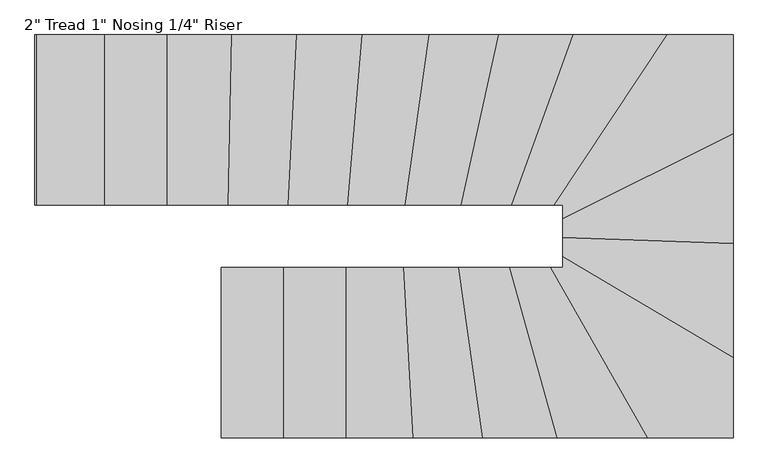
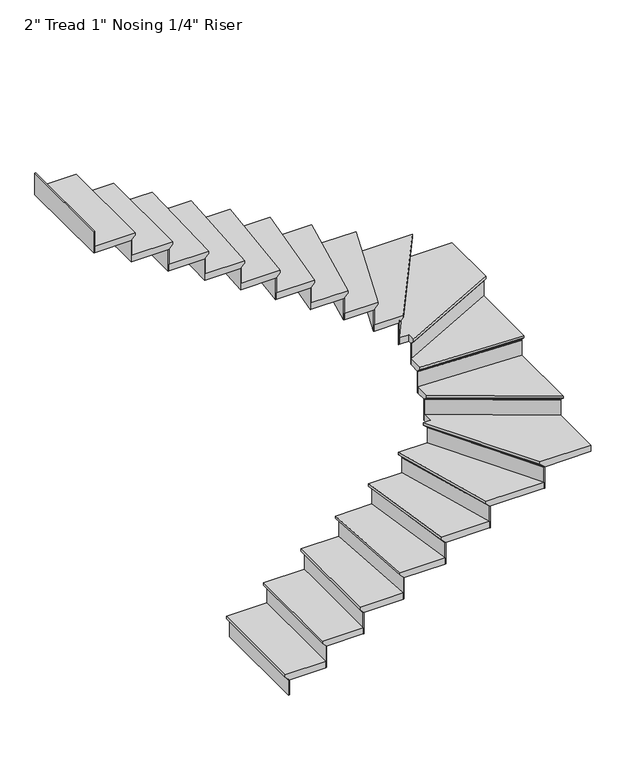
"""IFC4 building model written with IfcOpenShell, lengths in millimetres: stair flight geometry."""

from ifc_helpers import new_model, si_unit, origin, place, context, project, spatial, faceted_brep, source, transform, mapped, element, save


def stair_flight_7608b1ce(model_context):
    return source(origin(), model_context, "Body", "Brep", [
        faceted_brep([(3027.1038904, -664.1159676, 150.2833333), (3027.1038904, -664.1159676, 169.3333333), (3027.1038904, 97.8840324, 169.3333333), (3027.1038904, 97.8840324, 150.2833333), (3052.5038904, -664.1159676, 124.8833333), (3052.5038904, 97.8840324, 124.8833333), (3331.9038904, -664.1159676, 169.3333333), (3331.9038904, 97.8840324, 169.3333333), (3052.5038904, 97.8840324, 118.5333333), (3331.9038904, 97.8840324, 118.5333333), (3331.9038904, -664.1159676, 118.5333333), (3052.5038904, -664.1159676, 118.5333333)], [[[0, 1, 2, 3]], [[4, 0, 3, 5]], [[2, 1, 6, 7]], [[8, 9, 10, 11]], [[2, 7, 9, 8, 5, 3]], [[8, 11, 4, 5]], [[6, 1, 0, 4, 11, 10]], [[7, 6, 10, 9]]]),
        faceted_brep([(3052.5038904, -664.1159676, 118.5333333), (3052.5038904, -664.1159676, 0.0), (3058.8538904, -664.1159676, 0.0), (3058.8538904, -664.1159676, 118.5333333), (3052.5038904, 97.8840324, 118.5333333), (3058.8538904, 97.8840324, 118.5333333), (3058.8538904, 97.8840324, 0.0), (3052.5038904, 97.8840324, 0.0)], [[[0, 1, 2, 3]], [[4, 5, 6, 7]], [[1, 0, 4, 7]], [[2, 1, 7, 6]], [[3, 2, 6, 5]], [[0, 3, 5, 4]]]),
        faceted_brep([(3331.9038904, -664.1159676, 287.8666667), (3331.9038904, -664.1159676, 118.5333333), (3338.2538904, -664.1159676, 118.5333333), (3338.2538904, -664.1159676, 287.8666667), (3331.9038904, 97.8840324, 287.8666667), (3338.2538904, 97.8840324, 287.8666667), (3338.2538904, 97.8840324, 118.5333333), (3331.9038904, 97.8840324, 118.5333333)], [[[0, 1, 2, 3]], [[4, 5, 6, 7]], [[1, 0, 4, 7]], [[2, 1, 7, 6]], [[3, 2, 6, 5]], [[0, 3, 5, 4]]]),
        faceted_brep([(3306.5038904, 97.8840324, 338.6666667), (3306.5038904, -664.1159676, 338.6666667), (3611.3038904, -664.1159676, 338.6666667), (3611.3038904, 97.8840324, 338.6666667), (3331.9038904, 97.8840324, 287.8666667), (3611.3038904, 97.8840324, 287.8666667), (3611.3038904, -664.1159676, 287.8666667), (3331.9038904, -664.1159676, 287.8666667), (3331.9038904, 97.8840324, 294.2166667), (3306.5038904, 97.8840324, 319.6166667), (3331.9038904, -664.1159676, 294.2166667), (3306.5038904, -664.1159676, 319.6166667)], [[[0, 1, 2, 3]], [[4, 5, 6, 7]], [[0, 3, 5, 4, 8, 9]], [[4, 7, 10, 8]], [[2, 1, 11, 10, 7, 6]], [[3, 2, 6, 5]], [[11, 1, 0, 9]], [[10, 11, 9, 8]]]),
        faceted_brep([(3611.3038904, -664.1159676, 457.2), (3611.3038904, -664.1159676, 287.8666667), (3617.6538904, -664.1159676, 287.8666667), (3617.6538904, -664.1159676, 457.2), (3611.3038904, 97.8840324, 457.2), (3617.6538904, 97.8840324, 457.2), (3617.6538904, 97.8840324, 287.8666667), (3611.3038904, 97.8840324, 287.8666667)], [[[0, 1, 2, 3]], [[4, 5, 6, 7]], [[1, 0, 4, 7]], [[2, 1, 7, 6]], [[3, 2, 6, 5]], [[0, 3, 5, 4]]]),
        faceted_brep([(3585.9038904, 97.8840324, 508.0), (3585.9038904, -664.1159676, 508.0), (3912.204517, -664.1159676, 508.0), (3869.2837857, 97.8840324, 508.0), (3611.3038904, 97.8840324, 457.2), (3869.2837857, 97.8840324, 457.2), (3912.204517, -664.1159676, 457.2), (3611.3038904, -664.1159676, 457.2), (3611.3038904, 97.8840324, 463.55), (3585.9038904, 97.8840324, 488.95), (3611.3038904, -664.1159676, 463.55), (3585.9038904, -664.1159676, 488.95)], [[[0, 1, 2, 3]], [[4, 5, 6, 7]], [[0, 3, 5, 4, 8, 9]], [[4, 7, 10, 8]], [[2, 1, 11, 10, 7, 6]], [[3, 2, 6, 5]], [[11, 1, 0, 9]], [[10, 11, 9, 8]]]),
        faceted_brep([(3912.204517, -664.1159676, 626.5333333), (3912.204517, -664.1159676, 457.2), (3918.5645823, -664.1159676, 457.2), (3918.5645823, -664.1159676, 626.5333333), (3869.2837857, 97.8840324, 626.5333333), (3875.6438509, 97.8840324, 626.5333333), (3875.6438509, 97.8840324, 457.2), (3869.2837857, 97.8840324, 457.2)], [[[0, 1, 2, 3]], [[4, 5, 6, 7]], [[1, 0, 4, 7]], [[2, 1, 7, 6]], [[3, 2, 6, 5]], [[0, 3, 5, 4]]]),
        faceted_brep([(3843.8435247, 97.8840324, 677.3333333), (3886.7642561, -664.1159676, 677.3333333), (4223.9651309, -664.1159676, 677.3333333), (4116.7430968, 97.8840324, 677.3333333), (3869.2837857, 97.8840324, 626.5333333), (4116.7430968, 97.8840324, 626.5333333), (4223.9651309, -664.1159676, 626.5333333), (3912.204517, -664.1159676, 626.5333333), (3869.2837857, 97.8840324, 632.8833333), (3843.8435247, 97.8840324, 658.2833333), (3912.204517, -664.1159676, 632.8833333), (3886.7642561, -664.1159676, 658.2833333)], [[[0, 1, 2, 3]], [[4, 5, 6, 7]], [[0, 3, 5, 4, 8, 9]], [[4, 7, 10, 8]], [[2, 1, 11, 10, 7, 6]], [[3, 2, 6, 5]], [[11, 1, 0, 9]], [[10, 11, 9, 8]]]),
        faceted_brep([(4223.9651309, -664.1159676, 795.8666667), (4223.9651309, -664.1159676, 626.5333333), (4230.3776867, -664.1159676, 626.5333333), (4230.3776867, -664.1159676, 795.8666667), (4116.7430968, 97.8840324, 795.8666667), (4123.1556526, 97.8840324, 795.8666667), (4123.1556526, 97.8840324, 626.5333333), (4116.7430968, 97.8840324, 626.5333333)], [[[0, 1, 2, 3]], [[4, 5, 6, 7]], [[1, 0, 4, 7]], [[2, 1, 7, 6]], [[3, 2, 6, 5]], [[0, 3, 5, 4]]]),
        faceted_brep([(4091.0928734, 97.8840324, 846.6666667), (4198.3149075, -664.1159676, 846.6666667), (4557.577462, -664.1159676, 846.6666667), (4343.3988481, 97.8840324, 846.6666667), (4116.7430968, 97.8840324, 795.8666667), (4343.3988481, 97.8840324, 795.8666667), (4557.577462, -664.1159676, 795.8666667), (4223.9651309, -664.1159676, 795.8666667), (4116.7430968, 97.8840324, 802.2166667), (4091.0928734, 97.8840324, 827.6166667), (4223.9651309, -664.1159676, 802.2166667), (4198.3149075, -664.1159676, 827.6166667)], [[[0, 1, 2, 3]], [[4, 5, 6, 7]], [[0, 3, 5, 4, 8, 9]], [[4, 7, 10, 8]], [[2, 1, 11, 10, 7, 6]], [[3, 2, 6, 5]], [[11, 1, 0, 9]], [[10, 11, 9, 8]]]),
        faceted_brep([(4557.577462, -664.1159676, 965.2), (4557.577462, -664.1159676, 795.8666667), (4564.1735282, -664.1159676, 795.8666667), (4564.1735282, -664.1159676, 965.2), (4343.3988481, 97.8840324, 965.2), (4349.9949143, 97.8840324, 965.2), (4349.9949143, 97.8840324, 795.8666667), (4343.3988481, 97.8840324, 795.8666667)], [[[0, 1, 2, 3]], [[4, 5, 6, 7]], [[1, 0, 4, 7]], [[2, 1, 7, 6]], [[3, 2, 6, 5]], [[0, 3, 5, 4]]]),
        faceted_brep([(4317.0145835, 97.8840324, 1016.0), (4531.1931974, -664.1159676, 1016.0), (4964.5066423, -664.1159676, 1016.0), (4531.3858535, 97.8840324, 1016.0), (4343.3988481, 97.8840324, 965.2), (4531.3858535, 97.8840324, 965.2), (4964.5066423, -664.1159676, 965.2), (4557.577462, -664.1159676, 965.2), (4343.3988481, 97.8840324, 971.55), (4317.0145835, 97.8840324, 996.95), (4557.577462, -664.1159676, 971.55), (4531.1931974, -664.1159676, 996.95)], [[[0, 1, 2, 3]], [[4, 5, 6, 7]], [[0, 3, 5, 4, 8, 9]], [[4, 7, 10, 8]], [[2, 1, 11, 10, 7, 6]], [[3, 2, 6, 5]], [[11, 1, 0, 9]], [[10, 11, 9, 8]]]),
        faceted_brep([(4964.5066423, -664.1159676, 1134.5333333), (4964.5066423, -664.1159676, 965.2), (4971.8107395, -664.1159676, 965.2), (4971.8107395, -664.1159676, 1134.5333333), (4531.3858535, 97.8840324, 1134.5333333), (4538.6899506, 97.8840324, 1134.5333333), (4538.6899506, 97.8840324, 965.2), (4531.3858535, 97.8840324, 965.2)], [[[0, 1, 2, 3]], [[4, 5, 6, 7]], [[1, 0, 4, 7]], [[2, 1, 7, 6]], [[3, 2, 6, 5]], [[0, 3, 5, 4]]]),
        faceted_brep([(4554.8355823, 176.4983118, 1185.3333333), (4554.8355823, 97.8840324, 1185.3333333), (4502.1694651, 97.8840324, 1185.3333333), (4935.2902539, -664.1159676, 1185.3333333), (5316.8355823, -664.1159676, 1185.3333333), (5316.8355823, -274.7512133, 1185.3333333), (4554.8355823, 97.8840324, 1134.5333333), (4554.8355823, 176.4983118, 1134.5333333), (5316.8355823, -274.7512133, 1134.5333333), (5316.8355823, -664.1159676, 1134.5333333), (4964.5066423, -664.1159676, 1134.5333333), (4531.3858535, 97.8840324, 1134.5333333), (4531.3858535, 97.8840324, 1140.8833333), (4502.1694651, 97.8840324, 1166.2833333), (4964.5066423, -664.1159676, 1140.8833333), (4935.2902539, -664.1159676, 1166.2833333)], [[[0, 1, 2, 3, 4, 5]], [[6, 7, 8, 9, 10, 11]], [[1, 0, 7, 6]], [[2, 1, 6, 11, 12, 13]], [[11, 10, 14, 12]], [[4, 3, 15, 14, 10, 9]], [[5, 4, 9, 8]], [[0, 5, 8, 7]], [[15, 3, 2, 13]], [[14, 15, 13, 12]]]),
        faceted_brep([(5316.8355823, -274.7512133, 1303.8666667), (5316.8355823, -274.7512133, 1134.5333333), (5316.8355823, -267.3712943, 1134.5333333), (5316.8355823, -267.3712943, 1303.8666667), (4554.8355823, 176.4983118, 1303.8666667), (4554.8355823, 183.8782308, 1303.8666667), (4554.8355823, 183.8782308, 1134.5333333), (4554.8355823, 176.4983118, 1134.5333333)], [[[0, 1, 2, 3]], [[4, 5, 6, 7]], [[1, 0, 4, 7]], [[2, 1, 7, 6]], [[3, 2, 6, 5]], [[0, 3, 5, 4]]]),
        faceted_brep([(4554.8355823, 146.978636, 1354.6666667), (5316.8355823, -304.2708891, 1354.6666667), (5316.8355823, 231.0746698, 1354.6666667), (4554.8355823, 257.0661609, 1354.6666667), (4554.8355823, 176.4983118, 1303.8666667), (4554.8355823, 257.0661609, 1303.8666667), (5316.8355823, 231.0746698, 1303.8666667), (5316.8355823, -274.7512133, 1303.8666667), (4554.8355823, 176.4983118, 1310.2166667), (4554.8355823, 146.978636, 1335.6166667), (5316.8355823, -274.7512133, 1310.2166667), (5316.8355823, -304.2708891, 1335.6166667)], [[[0, 1, 2, 3]], [[4, 5, 6, 7]], [[0, 3, 5, 4, 8, 9]], [[4, 7, 10, 8]], [[3, 2, 6, 5]], [[11, 1, 0, 9]], [[10, 11, 9, 8]], [[2, 1, 11, 10, 7, 6]]]),
        faceted_brep([(5316.8355823, 231.0746698, 1473.2), (5316.8355823, 231.0746698, 1303.8666667), (5316.8355823, 237.4283627, 1303.8666667), (5316.8355823, 237.4283627, 1473.2), (4554.8355823, 257.0661609, 1473.2), (4554.8355823, 263.4198538, 1473.2), (4554.8355823, 263.4198538, 1303.8666667), (4554.8355823, 257.0661609, 1303.8666667)], [[[0, 1, 2, 3]], [[4, 5, 6, 7]], [[1, 0, 4, 7]], [[2, 1, 7, 6]], [[3, 2, 6, 5]], [[0, 3, 5, 4]]]),
        faceted_brep([(4554.8355823, 231.6513892, 1524.0), (5316.8355823, 205.6598981, 1524.0), (5316.8355823, 725.540021, 1524.0), (4554.8355823, 345.3712777, 1524.0), (4554.8355823, 257.0661609, 1473.2), (4554.8355823, 345.3712777, 1473.2), (5316.8355823, 725.540021, 1473.2), (5316.8355823, 231.0746698, 1473.2), (4554.8355823, 257.0661609, 1479.55), (4554.8355823, 231.6513892, 1504.95), (5316.8355823, 231.0746698, 1479.55), (5316.8355823, 205.6598981, 1504.95)], [[[0, 1, 2, 3]], [[4, 5, 6, 7]], [[0, 3, 5, 4, 8, 9]], [[4, 7, 10, 8]], [[2, 1, 11, 10, 7, 6]], [[3, 2, 6, 5]], [[11, 1, 0, 9]], [[10, 11, 9, 8]]]),
        faceted_brep([(5316.8355823, 725.540021, 1642.5333333), (5316.8355823, 725.540021, 1473.2), (5316.8355823, 732.6364416, 1473.2), (5316.8355823, 732.6364416, 1642.5333333), (4554.8355823, 345.3712777, 1642.5333333), (4554.8355823, 352.4676983, 1642.5333333), (4554.8355823, 352.4676983, 1473.2), (4554.8355823, 345.3712777, 1473.2)], [[[0, 1, 2, 3]], [[4, 5, 6, 7]], [[1, 0, 4, 7]], [[2, 1, 7, 6]], [[3, 2, 6, 5]], [[0, 3, 5, 4]]]),
        faceted_brep([(4485.0145037, 377.2840324, 1693.3333333), (4554.8355823, 377.2840324, 1693.3333333), (4554.8355823, 316.9855952, 1693.3333333), (5316.8355823, 697.1543385, 1693.3333333), (5316.8355823, 1139.2840324, 1693.3333333), (4990.2073577, 1139.2840324, 1693.3333333), (4554.8355823, 377.2840324, 1642.5333333), (4485.0145037, 377.2840324, 1642.5333333), (4990.2073577, 1139.2840324, 1642.5333333), (5316.8355823, 1139.2840324, 1642.5333333), (5316.8355823, 725.540021, 1642.5333333), (4554.8355823, 345.3712777, 1642.5333333), (5316.8355823, 725.540021, 1648.8833333), (4554.8355823, 345.3712777, 1648.8833333), (5316.8355823, 697.1543385, 1674.2833333), (4554.8355823, 316.9855952, 1674.2833333)], [[[0, 1, 2, 3, 4, 5]], [[6, 7, 8, 9, 10, 11]], [[1, 0, 7, 6]], [[11, 10, 12, 13]], [[4, 3, 14, 12, 10, 9]], [[5, 4, 9, 8]], [[0, 5, 8, 7]], [[14, 3, 2, 15]], [[12, 14, 15, 13]], [[2, 1, 6, 11, 13, 15]]]),
        faceted_brep([(4990.2073577, 1139.2840324, 1811.8666667), (4990.2073577, 1139.2840324, 1642.5333333), (4982.5885587, 1139.2840324, 1642.5333333), (4982.5885587, 1139.2840324, 1811.8666667), (4485.0145037, 377.2840324, 1811.8666667), (4477.3957047, 377.2840324, 1811.8666667), (4477.3957047, 377.2840324, 1642.5333333), (4485.0145037, 377.2840324, 1642.5333333)], [[[0, 1, 2, 3]], [[4, 5, 6, 7]], [[1, 0, 4, 7]], [[2, 1, 7, 6]], [[3, 2, 6, 5]], [[0, 3, 5, 4]]]),
        faceted_brep([(4515.4896998, 377.2840324, 1862.6666667), (5020.6825538, 1139.2840324, 1862.6666667), (4571.9006048, 1139.2840324, 1862.6666667), (4297.6089866, 377.2840324, 1862.6666667), (4485.0145037, 377.2840324, 1811.8666667), (4297.6089866, 377.2840324, 1811.8666667), (4571.9006048, 1139.2840324, 1811.8666667), (4990.2073577, 1139.2840324, 1811.8666667), (4485.0145037, 377.2840324, 1818.2166667), (4515.4896998, 377.2840324, 1843.6166667), (4990.2073577, 1139.2840324, 1818.2166667), (5020.6825538, 1139.2840324, 1843.6166667)], [[[0, 1, 2, 3]], [[4, 5, 6, 7]], [[0, 3, 5, 4, 8, 9]], [[4, 7, 10, 8]], [[2, 1, 11, 10, 7, 6]], [[3, 2, 6, 5]], [[11, 1, 0, 9]], [[10, 11, 9, 8]]]),
        faceted_brep([(4571.9006048, 1139.2840324, 1981.2), (4571.9006048, 1139.2840324, 1811.8666667), (4565.1517372, 1139.2840324, 1811.8666667), (4565.1517372, 1139.2840324, 1981.2), (4297.6089866, 377.2840324, 1981.2), (4290.8601189, 377.2840324, 1981.2), (4290.8601189, 377.2840324, 1811.8666667), (4297.6089866, 377.2840324, 1811.8666667)], [[[0, 1, 2, 3]], [[4, 5, 6, 7]], [[1, 0, 4, 7]], [[2, 1, 7, 6]], [[3, 2, 6, 5]], [[0, 3, 5, 4]]]),
        faceted_brep([(4324.6044572, 377.2840324, 2032.0), (4598.8960755, 1139.2840324, 2032.0), (4240.5068778, 1139.2840324, 2032.0), (4072.1688015, 377.2840324, 2032.0), (4297.6089866, 377.2840324, 1981.2), (4072.1688015, 377.2840324, 1981.2), (4240.5068778, 1139.2840324, 1981.2), (4571.9006048, 1139.2840324, 1981.2), (4297.6089866, 377.2840324, 1987.55), (4324.6044572, 377.2840324, 2012.95), (4571.9006048, 1139.2840324, 1987.55), (4598.8960755, 1139.2840324, 2012.95)], [[[0, 1, 2, 3]], [[4, 5, 6, 7]], [[0, 3, 5, 4, 8, 9]], [[4, 7, 10, 8]], [[2, 1, 11, 10, 7, 6]], [[3, 2, 6, 5]], [[11, 1, 0, 9]], [[10, 11, 9, 8]]]),
        faceted_brep([(4240.5068778, 1139.2840324, 2150.5333333), (4240.5068778, 1139.2840324, 1981.2), (4234.0037712, 1139.2840324, 1981.2), (4234.0037712, 1139.2840324, 2150.5333333), (4072.1688015, 377.2840324, 2150.5333333), (4065.6656948, 377.2840324, 2150.5333333), (4065.6656948, 377.2840324, 1981.2), (4072.1688015, 377.2840324, 1981.2)], [[[0, 1, 2, 3]], [[4, 5, 6, 7]], [[1, 0, 4, 7]], [[2, 1, 7, 6]], [[3, 2, 6, 5]], [[0, 3, 5, 4]]]),
        faceted_brep([(4098.1812282, 377.2840324, 2201.3333333), (4266.5193045, 1139.2840324, 2201.3333333), (3930.5940796, 1139.2840324, 2201.3333333), (3824.011933, 377.2840324, 2201.3333333), (4072.1688015, 377.2840324, 2150.5333333), (3824.011933, 377.2840324, 2150.5333333), (3930.5940796, 1139.2840324, 2150.5333333), (4240.5068778, 1139.2840324, 2150.5333333), (4072.1688015, 377.2840324, 2156.8833333), (4098.1812282, 377.2840324, 2182.2833333), (4240.5068778, 1139.2840324, 2156.8833333), (4266.5193045, 1139.2840324, 2182.2833333)], [[[0, 1, 2, 3]], [[4, 5, 6, 7]], [[0, 3, 5, 4, 8, 9]], [[4, 7, 10, 8]], [[2, 1, 11, 10, 7, 6]], [[3, 2, 6, 5]], [[11, 1, 0, 9]], [[10, 11, 9, 8]]]),
        faceted_brep([(3930.5940796, 1139.2840324, 2319.8666667), (3930.5940796, 1139.2840324, 2150.5333333), (3924.1822646, 1139.2840324, 2150.5333333), (3924.1822646, 1139.2840324, 2319.8666667), (3824.011933, 377.2840324, 2319.8666667), (3817.600118, 377.2840324, 2319.8666667), (3817.600118, 377.2840324, 2150.5333333), (3824.011933, 377.2840324, 2150.5333333)], [[[0, 1, 2, 3]], [[4, 5, 6, 7]], [[1, 0, 4, 7]], [[2, 1, 7, 6]], [[3, 2, 6, 5]], [[0, 3, 5, 4]]]),
        faceted_brep([(3849.659193, 377.2840324, 2370.6666667), (3956.2413397, 1139.2840324, 2370.6666667), (3631.1254825, 1139.2840324, 2370.6666667), (3564.9840405, 377.2840324, 2370.6666667), (3824.011933, 377.2840324, 2319.8666667), (3564.9840405, 377.2840324, 2319.8666667), (3631.1254825, 1139.2840324, 2319.8666667), (3930.5940796, 1139.2840324, 2319.8666667), (3824.011933, 377.2840324, 2326.2166667), (3849.659193, 377.2840324, 2351.6166667), (3930.5940796, 1139.2840324, 2326.2166667), (3956.2413397, 1139.2840324, 2351.6166667)], [[[0, 1, 2, 3]], [[4, 5, 6, 7]], [[0, 3, 5, 4, 8, 9]], [[4, 7, 10, 8]], [[2, 1, 11, 10, 7, 6]], [[3, 2, 6, 5]], [[11, 1, 0, 9]], [[10, 11, 9, 8]]]),
        faceted_brep([(3631.1254825, 1139.2840324, 2489.2), (3631.1254825, 1139.2840324, 2319.8666667), (3624.7516063, 1139.2840324, 2319.8666667), (3624.7516063, 1139.2840324, 2489.2), (3564.9840405, 377.2840324, 2489.2), (3558.6101643, 377.2840324, 2489.2), (3558.6101643, 377.2840324, 2319.8666667), (3564.9840405, 377.2840324, 2319.8666667)], [[[0, 1, 2, 3]], [[4, 5, 6, 7]], [[1, 0, 4, 7]], [[2, 1, 7, 6]], [[3, 2, 6, 5]], [[0, 3, 5, 4]]]),
        faceted_brep([(3590.4795453, 377.2840324, 2540.0), (3656.6209874, 1139.2840324, 2540.0), (3337.5216683, 1139.2840324, 2540.0), (3299.9170425, 377.2840324, 2540.0), (3564.9840405, 377.2840324, 2489.2), (3299.9170425, 377.2840324, 2489.2), (3337.5216683, 1139.2840324, 2489.2), (3631.1254825, 1139.2840324, 2489.2), (3564.9840405, 377.2840324, 2495.55), (3590.4795453, 377.2840324, 2520.95), (3631.1254825, 1139.2840324, 2495.55), (3656.6209874, 1139.2840324, 2520.95)], [[[0, 1, 2, 3]], [[4, 5, 6, 7]], [[0, 3, 5, 4, 8, 9]], [[4, 7, 10, 8]], [[2, 1, 11, 10, 7, 6]], [[3, 2, 6, 5]], [[11, 1, 0, 9]], [[10, 11, 9, 8]]]),
        faceted_brep([(3337.5216683, 1139.2840324, 2658.5333333), (3337.5216683, 1139.2840324, 2489.2), (3331.1639406, 1139.2840324, 2489.2), (3331.1639406, 1139.2840324, 2658.5333333), (3299.9170425, 377.2840324, 2658.5333333), (3293.5593148, 377.2840324, 2658.5333333), (3293.5593148, 377.2840324, 2489.2), (3299.9170425, 377.2840324, 2489.2)], [[[0, 1, 2, 3]], [[4, 5, 6, 7]], [[1, 0, 4, 7]], [[2, 1, 7, 6]], [[3, 2, 6, 5]], [[0, 3, 5, 4]]]),
        faceted_brep([(3325.3479534, 377.2840324, 2709.3333333), (3362.9525793, 1139.2840324, 2709.3333333), (3047.5394266, 1139.2840324, 2709.3333333), (3031.1493561, 377.2840324, 2709.3333333), (3299.9170425, 377.2840324, 2658.5333333), (3031.1493561, 377.2840324, 2658.5333333), (3047.5394266, 1139.2840324, 2658.5333333), (3337.5216683, 1139.2840324, 2658.5333333), (3299.9170425, 377.2840324, 2664.8833333), (3325.3479534, 377.2840324, 2690.2833333), (3337.5216683, 1139.2840324, 2664.8833333), (3362.9525793, 1139.2840324, 2690.2833333)], [[[0, 1, 2, 3]], [[4, 5, 6, 7]], [[0, 3, 5, 4, 8, 9]], [[4, 7, 10, 8]], [[2, 1, 11, 10, 7, 6]], [[3, 2, 6, 5]], [[11, 1, 0, 9]], [[10, 11, 9, 8]]]),
        faceted_brep([(3047.5394266, 1139.2840324, 2827.8666667), (3047.5394266, 1139.2840324, 2658.5333333), (3041.1879579, 1139.2840324, 2658.5333333), (3041.1879579, 1139.2840324, 2827.8666667), (3031.1493561, 377.2840324, 2827.8666667), (3024.7978874, 377.2840324, 2827.8666667), (3024.7978874, 377.2840324, 2658.5333333), (3031.1493561, 377.2840324, 2658.5333333)], [[[0, 1, 2, 3]], [[4, 5, 6, 7]], [[1, 0, 4, 7]], [[2, 1, 7, 6]], [[3, 2, 6, 5]], [[0, 3, 5, 4]]]),
        faceted_brep([(3056.5552311, 377.2840324, 2878.6666667), (3072.9453016, 1139.2840324, 2878.6666667), (2759.9502663, 1139.2840324, 2878.6666667), (2759.9502663, 377.2840324, 2878.6666667), (3031.1493561, 377.2840324, 2827.8666667), (2759.9502663, 377.2840324, 2827.8666667), (2759.9502663, 1139.2840324, 2827.8666667), (3047.5394266, 1139.2840324, 2827.8666667), (3031.1493561, 377.2840324, 2834.2166667), (3056.5552311, 377.2840324, 2859.6166667), (3047.5394266, 1139.2840324, 2834.2166667), (3072.9453016, 1139.2840324, 2859.6166667)], [[[0, 1, 2, 3]], [[4, 5, 6, 7]], [[0, 3, 5, 4, 8, 9]], [[4, 7, 10, 8]], [[2, 1, 11, 10, 7, 6]], [[3, 2, 6, 5]], [[11, 1, 0, 9]], [[10, 11, 9, 8]]]),
        faceted_brep([(2759.9502663, 1139.2840324, 2997.2), (2759.9502663, 1139.2840324, 2827.8666667), (2753.6002663, 1139.2840324, 2827.8666667), (2753.6002663, 1139.2840324, 2997.2), (2759.9502663, 377.2840324, 2997.2), (2753.6002663, 377.2840324, 2997.2), (2753.6002663, 377.2840324, 2827.8666667), (2759.9502663, 377.2840324, 2827.8666667)], [[[0, 1, 2, 3]], [[4, 5, 6, 7]], [[1, 0, 4, 7]], [[2, 1, 7, 6]], [[3, 2, 6, 5]], [[0, 3, 5, 4]]]),
        faceted_brep([(2785.3502663, 377.2840324, 3048.0), (2785.3502663, 1139.2840324, 3048.0), (2480.5502663, 1139.2840324, 3048.0), (2480.5502663, 377.2840324, 3048.0), (2759.9502663, 377.2840324, 2997.2), (2480.5502663, 377.2840324, 2997.2), (2480.5502663, 1139.2840324, 2997.2), (2759.9502663, 1139.2840324, 2997.2), (2759.9502663, 377.2840324, 3003.55), (2785.3502663, 377.2840324, 3028.95), (2759.9502663, 1139.2840324, 3003.55), (2785.3502663, 1139.2840324, 3028.95)], [[[0, 1, 2, 3]], [[4, 5, 6, 7]], [[0, 3, 5, 4, 8, 9]], [[4, 7, 10, 8]], [[2, 1, 11, 10, 7, 6]], [[3, 2, 6, 5]], [[11, 1, 0, 9]], [[10, 11, 9, 8]]]),
        faceted_brep([(2480.5502663, 1139.2840324, 3166.5333333), (2480.5502663, 1139.2840324, 2997.2), (2474.2002663, 1139.2840324, 2997.2), (2474.2002663, 1139.2840324, 3166.5333333), (2480.5502663, 377.2840324, 3166.5333333), (2474.2002663, 377.2840324, 3166.5333333), (2474.2002663, 377.2840324, 2997.2), (2480.5502663, 377.2840324, 2997.2)], [[[0, 1, 2, 3]], [[4, 5, 6, 7]], [[1, 0, 4, 7]], [[2, 1, 7, 6]], [[3, 2, 6, 5]], [[0, 3, 5, 4]]]),
        faceted_brep([(2201.1502663, 1139.2840324, 3335.8666667), (2201.1502663, 1139.2840324, 3166.5333333), (2194.8002663, 1139.2840324, 3166.5333333), (2194.8002663, 1139.2840324, 3335.8666667), (2201.1502663, 377.2840324, 3335.8666667), (2194.8002663, 377.2840324, 3335.8666667), (2194.8002663, 377.2840324, 3166.5333333), (2201.1502663, 377.2840324, 3166.5333333)], [[[0, 1, 2, 3]], [[4, 5, 6, 7]], [[1, 0, 4, 7]], [[2, 1, 7, 6]], [[3, 2, 6, 5]], [[0, 3, 5, 4]]]),
        faceted_brep([(2505.9502663, 377.2840324, 3217.3333333), (2505.9502663, 1139.2840324, 3217.3333333), (2201.1502663, 1139.2840324, 3217.3333333), (2201.1502663, 377.2840324, 3217.3333333), (2480.5502663, 377.2840324, 3166.5333333), (2201.1502663, 377.2840324, 3166.5333333), (2201.1502663, 1139.2840324, 3166.5333333), (2480.5502663, 1139.2840324, 3166.5333333), (2480.5502663, 377.2840324, 3172.8833333), (2505.9502663, 377.2840324, 3198.2833333), (2480.5502663, 1139.2840324, 3172.8833333), (2505.9502663, 1139.2840324, 3198.2833333)], [[[0, 1, 2, 3]], [[4, 5, 6, 7]], [[0, 3, 5, 4, 8, 9]], [[4, 7, 10, 8]], [[2, 1, 11, 10, 7, 6]], [[3, 2, 6, 5]], [[11, 1, 0, 9]], [[10, 11, 9, 8]]]),
    ])


if __name__ == "__main__":
    model = new_model("IFC4")
    model_context = context("Model", 3, world=origin())
    ifc_project = project(units=[si_unit("LENGTHUNIT", "METRE", prefix="MILLI")], contexts=[model_context])
    site = spatial("IfcSite", under=ifc_project)
    building = spatial("IfcBuilding", under=site)
    placement = place(None, origin())
    stair_flight_shape = stair_flight_7608b1ce(model_context)
    element("IfcStairFlight", 1, ObjectType="2\" Tread 1\" Nosing 1/4\" Riser", at=placement, inside=building, context=model_context, shape_type="MappedRepresentation", body=[
        mapped(stair_flight_shape, transform((0.0, 0.0, 0.0), x_axis=(1.0, 0.0, 0.0), y_axis=(0.0, 1.0, 0.0), z_axis=(0.0, 0.0, 1.0))),
    ])
    save(model, "model.ifc")
